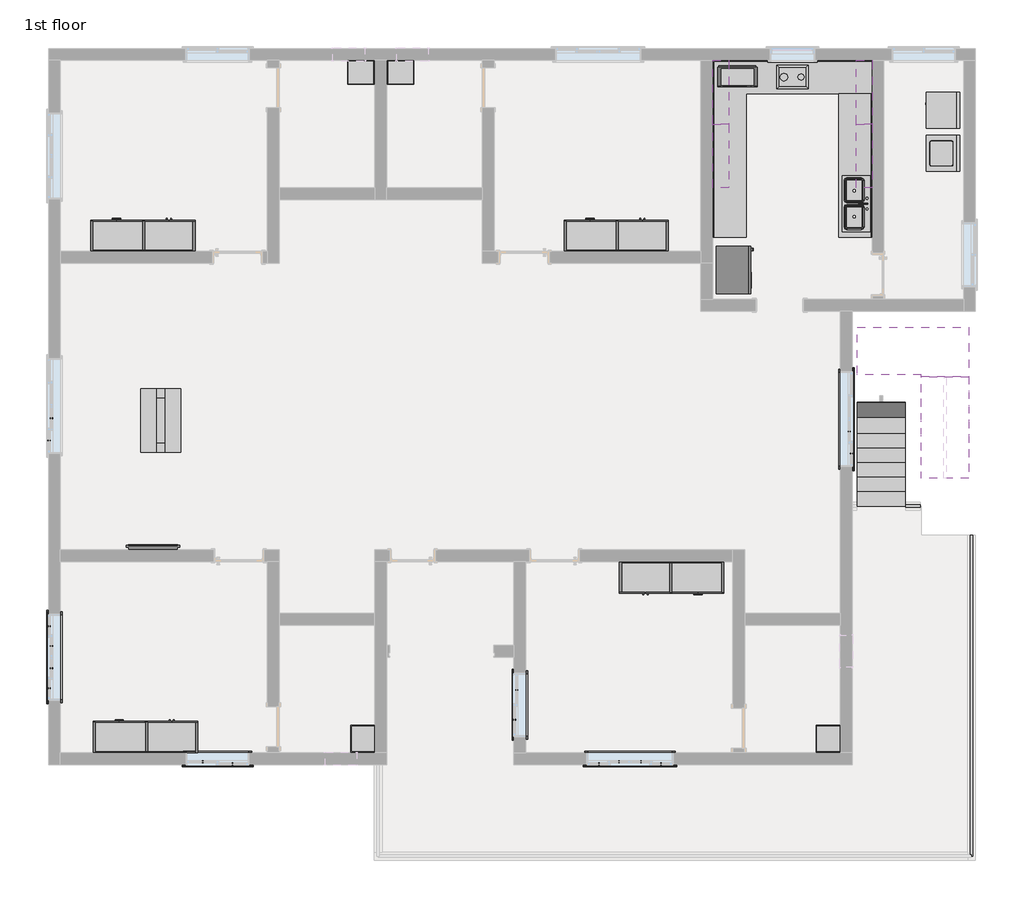
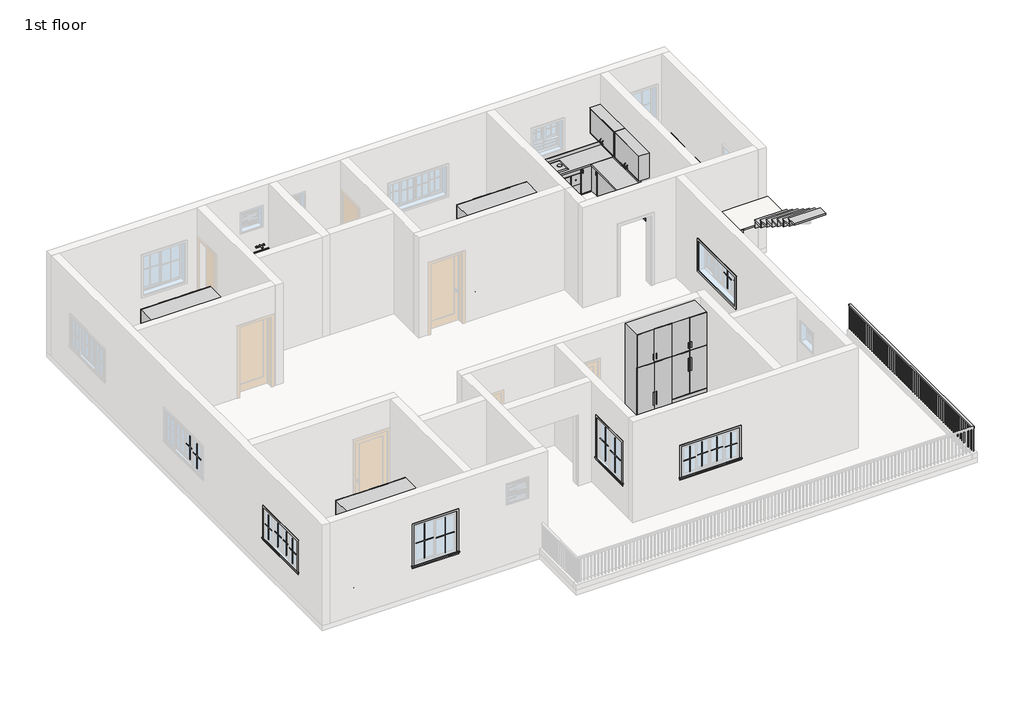
# One storey, part 3 of 4: 30 proxies, 19 furniture elements, 5 flow terminals, 2 railings, 2 stair flights, 1 slab.
# Revit data of these elements (continued)
# Elements 23, 24 (IfcBuildingElementProxy, "Trim-Window-Exterior-Flat : with Sill") (continued)
#   Opening Width = 4' - 0"
#   Opening Height = 4' - 0"
#   Trim Material = Clad - White
#   Phase Created = New Construction
#   Materials on its faces: "Clad - White"
# Elements 25, 26 (IfcBuildingElementProxy, "Trim-Window-Interior-Flat : Picture Frame")
#   Opening Width = 5' - 5"
#   Opening Height = 3' - 0"
#   Trim Material = Wood - Stained
#   Phase Created = New Construction
#   Materials on its faces: "Wood - Stained"
# Element 27 (IfcBuildingElementProxy, "Trim-Window-Interior-Flat : Picture Frame")
#   Opening Width = 6' - 0"
#   Opening Height = 3' - 0"
#   Trim Material = Wood - Stained
#   Phase Created = New Construction
#   Materials on its faces: "Wood - Stained"
# Elements 28, 29 (IfcBuildingElementProxy, "Trim-Window-Interior-Flat : Picture Frame")
#   Opening Width = 4' - 0"
#   Opening Height = 4' - 0"
#   Trim Material = Wood - Stained
#   Phase Created = New Construction
#   Materials on its faces: "Wood - Stained"
# Element 30 (IfcBuildingElementProxy, "Washer : 27\" x 25\" x 35\"")
#   Phase Created = New Construction
#   Materials on its faces: "Metal - Paint Finish - Ivory,Matte"
# Element 31 (IfcFlowTerminal, "Sink - Work : 20\"x18\"")
#   Mark = "19"
#   Flow Pressure = 8.00 psi
#   Phase Created = New Construction
# Element 32 (IfcFlowTerminal, "Sink - Work : 20\"x18\"")
#   Mark = "20"
#   Flow Pressure = 8.00 psi
#   Phase Created = New Construction
# Element 33 (IfcFlowTerminal, "Sink - Work : 20\"x18\"")
#   Mark = "21"
#   Flow Pressure = 8.00 psi
#   Phase Created = New Construction
# Element 34 (IfcFlowTerminal, "Sink - Work : 20\"x18\"")
#   Mark = "22"
#   Flow Pressure = 8.00 psi
#   Phase Created = New Construction
# Element 35 (IfcFlowTerminal, "Sink Kitchen-Double : 42\" x 21\"")
#   Mark = "14"
#   Phase Created = New Construction
#   Materials on its faces: "Steel, Polished"
# Element 36 (IfcFurniture)
#   Phase Created = New Construction
#   Materials on its faces: "Default", "Default 3", "Default 2"
# Elements 37, 38, 39, 40 (IfcFurniture, "1Wardrobe_6271 : 1Wardrobe_6271")
#   Phase Created = New Construction
#   Materials on its faces: "Phase - Demo", "Default Wall", "Phase - Exist", "Default"
# Elements 41, 42, 43, 44 (IfcFurniture, "48\" 2")
#   Phase Created = New Construction
#   Materials on its faces: "Cabinets", "Cabinets - Handles"
# Elements 45, 46 (IfcFurniture, "Base Cabinet-Corner Unit-Square : 36\"")
#   Phase Created = New Construction
#   Materials on its faces: "Cabinets", "Cabinets - Handles"
# Element 47 (IfcFurniture, "Counter Top w Sink : 24\" Depth")
#   Sink Opening Width = 3' - 3"
#   Sink Opening Depth = 1' - 3"
#   Sink Location To Wall = 0' - 6"
#   Sink Location = 6' - 11"
#   Length = 9' - 0.36336"
#   Phase Created = New Construction
#   Materials on its faces: "Counter Top"
# Element 48 (IfcFurniture, "Counter Top-L Shaped : 24\" Depth")
#   Length - Leg 2 = 11' - 1.36336"
#   Length - Leg 1 = 10' - 0"
#   Phase Created = New Construction
#   Materials on its faces: "Counter Top"
# Element 49 (IfcFurniture, "Television-Plasma : 42\"")
#   Phase Created = New Construction
#   Materials on its faces: "Plastic - Gray", "Glass"
# Elements 50, 51, 52, 53 (IfcFurniture, "Upper Cabinet-Pass-Thru : 48\" x 30\" x 12\"")
#   Phase Created = New Construction
#   Materials on its faces: "Cabinet"
# Element 54 (IfcFurniture, "White_Modern_Coffee_Table_17067 : White_Modern_Coffee_Table_17067")
#   Phase Created = New Construction
#   Materials on its faces: "White Modern Coffee Table - Plastic", "White Modern Coffee Table - Wood"
# Elements 55, 56 (IfcRailing, "Handrail - Rectangular")
#   Phase Created = New Construction
# Element 57 (IfcSlab, "Non-Monolithic Landing")
#   Phase Created = New Construction
# Elements 58, 59 (IfcStairFlight, "2\" Tread 1\" Nosing 1/4\" Riser")
#   Phase Created = New Construction
# Materials
#   "Metal - Chrome": colour RGB 17 17 17, transparency 0
#   "Metal - Steel, Polished": colour RGB 57 57 57, transparency 0
#   "Metal - Paint Finish - Ivory,Glossy": colour RGB 247 247 239, transparency 0
#   "Laminate - Ivory,Matte": colour RGB 247 247 239, transparency 0
#   "Metal - Paint Finish - Ivory,Matte": colour RGB 247 247 239, transparency 0
#   "Steel, Polished": class "Metal", colour RGB 192 192 192, transparency 0, Description = "Polished steel", Cost = 0
#   "Cabinets - Handles": class "Metal", colour RGB 57 57 57, transparency 0
#   "Cabinets": colour RGB 249 249 249, transparency 0
#   "Plastic - Gray": colour RGB 134 134 134, transparency 0
#   "White Modern Coffee Table - Wood": class "Generic", colour RGB 120 120 120, transparency 0, Cost = 0
#   "White Modern Coffee Table - Plastic": class "Generic", colour RGB 120 120 120, transparency 0, Cost = 0
#   "Glass": class "Glass", colour RGB 0 128 192, transparency 0.75, Description = "Soda Lime Glass", Cost = 0
#   "Clad - White": class "Wood", colour RGB 242 242 238, transparency 0, Cost = 0
#   "Wood - Stained": class "Wood", colour RGB 224 178 126, transparency 0, Cost = 0
#   "Default": colour RGB 127 127 127, transparency 0, Cost = 0
#   "Default 3": class "Glass", colour RGB 127 127 127, transparency 0
#   "Default 2": class "Plastic", colour RGB 127 127 127, transparency 0
#   "Phase - Demo": class "System", colour RGB 255 0 0, transparency 0.4, Cost = 0
#   "Default Wall": colour RGB 128 128 128, transparency 0, Cost = 0
#   "Phase - Exist": class "System", colour RGB 127 127 127, transparency 0, Cost = 0
#   "Counter Top": class "Wood", colour RGB 226 177 128, transparency 0
#   "Cabinet": colour RGB 204 122 2, transparency 0
